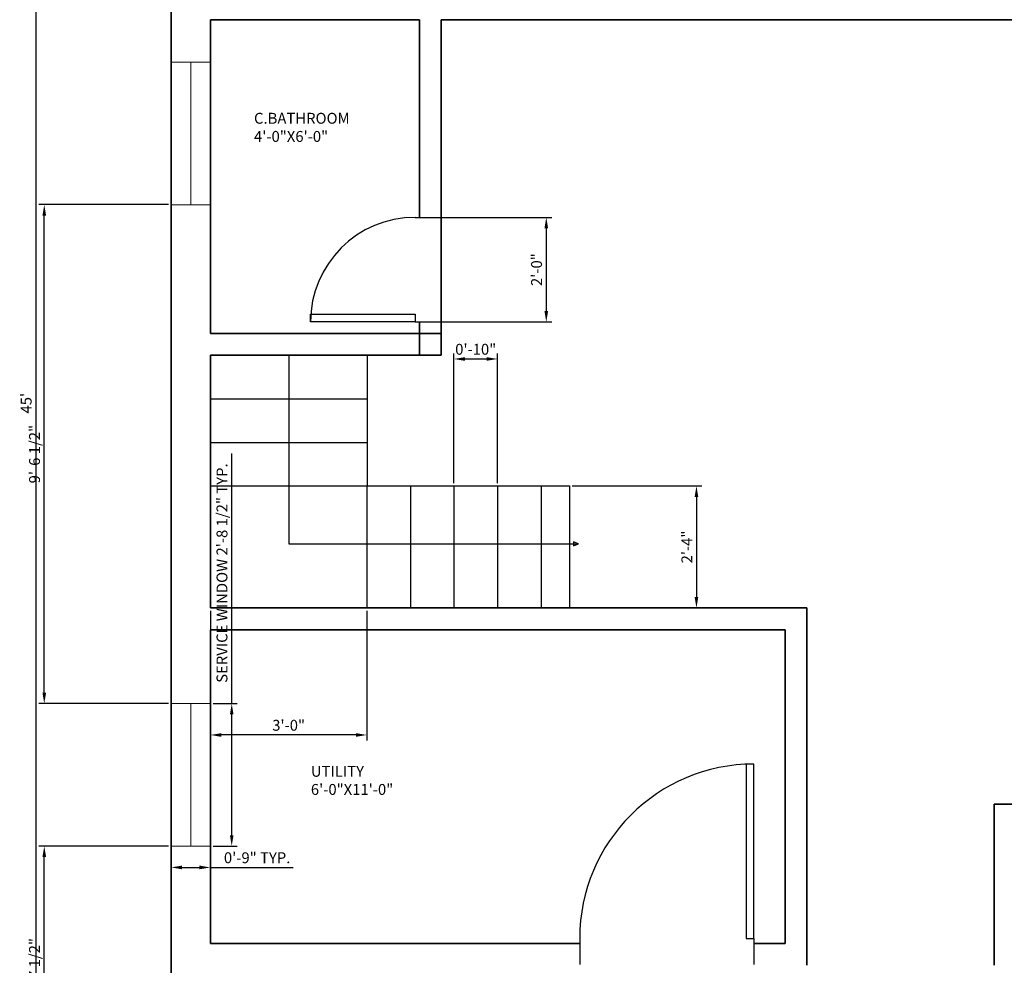
# Model space of a CAD drawing. Units: inches. Extents: x 2981 to 3526, y 1512 to 2158.
# Tile 2 of 4: x 2981 to 3207, y 1713 to 1930. Entities that reach past the tile are written whole.
import ezdxf

# ---------------------------------------------------------------- set-up
doc = ezdxf.new("R2010")
doc.units = ezdxf.units.IN
for name, color, linetype, lineweight in [('A-ANNO-DIMS', 2, 'Continuous', 18), ('A-AREA-IDEN', 7, 'Continuous', 18), ('A-DOOR', 4, 'Continuous', 25), ('A-FLOR-STRS', 7, 'Continuous', 25), ('A-GLAZ', 4, 'Continuous', 18), ('A-WALL', 7, 'Continuous', 35)]:
    doc.layers.add(name, color=color, linetype=linetype, lineweight=lineweight)
doc.styles.get("Standard").update_dxf_attribs({"font": 'arial.ttf'})
doc.dimstyles.new('ISO-25', dxfattribs={"dimtxt": 2.5, "dimasz": 2.5, "dimexe": 1.25, "dimexo": 0.625, "dimtad": 1, "dimlunit": 3, "dimtxsty": 'Standard', "dimcen": 2.5, "dimadec": 0, "dimazin": 0, "dimtfac": 1, "dimtmove": 0, "dimatfit": 3, "dimfxl": 1, "dimarcsym": 0})

# ---------------------------------------------------------------- blocks, each defined once
blk = doc.blocks.new('*U5')
for p, q in [((0, 0), (0, -6)), ((24, 0), (24, -6))]:
    blk.add_line(p, q)
blk.add_lwpolyline([(0, 0), (0, 24), (1.75, 24), (1.75, 0)], close=True)
blk.add_arc((0, 0), 24, 0, 90)
blk = doc.blocks.new('*U4')
for p, q in [((0, 0), (0, -6)), ((-40, 0), (-40, -6))]:
    blk.add_line(p, q)
blk.add_lwpolyline([(0, 0), (0, 40), (-1.75, 40), (-1.75, 0)], close=True)
blk.add_arc((0, 0), 40, 90, 180)
blk = doc.blocks.new('*D15')
at = {"layer": 'A-ANNO-DIMS', "color": 0, "lineweight": -2, "transparency": 16777216}
for p, q in [((3014.77, 2112.2), (2983.05, 2112.2)), ((2984.3, 2109.7), (2984.3, 1574.7)), ((3014.77, 1572.2), (2983.05, 1572.2))]:
    blk.add_line(p, q, dxfattribs=at)
at = {"layer": 'A-ANNO-DIMS', "color": 0, "transparency": 16777216}
for points in [[(2983.89, 2109.7), (2984.72, 2109.7), (2984.3, 2112.2)], [(2983.89, 1574.7), (2984.72, 1574.7), (2984.3, 1572.2)]]:
    blk.add_solid(points, dxfattribs=at)
at = {"layer": 'Defpoints', "color": 0, "transparency": 16777216}
for p in [(3015.4, 2112.2), (2984.3, 1572.2), (3015.4, 1572.2)]:
    blk.add_point(p, dxfattribs=at)
at = {"layer": 'A-ANNO-DIMS', "color": 0, "transparency": 16777216, "insert": (2982.41, 1842.2), "char_height": 2.5, "attachment_point": 5, "rotation": 90}
blk.add_mtext("45'", dxfattribs=at)
blk = doc.blocks.new('WIN-33IN-SERVICE')
for p, q in [((9, 32.7), (0, 32.7)), ((0, 32.7), (0, 0)), ((9, 32.7), (4.5, 32.7)), ((4.5, 32.7), (4.5, 0)), ((9, 0), (9, 32.7)), ((0, 0), (9, 0))]:
    blk.add_line(p, q)
blk = doc.blocks.new('*D33')
at = {"layer": 'A-ANNO-DIMS', "color": 0, "lineweight": -2, "transparency": 16777216}
for p, q in [((3029.3, 1773.26), (3029.3, 1830.66)), ((3025.02, 1773.26), (3030.55, 1773.26)), ((3029.3, 1743.06), (3029.3, 1770.76)), ((3025.02, 1740.56), (3030.55, 1740.56))]:
    blk.add_line(p, q, dxfattribs=at)
at = {"layer": 'A-ANNO-DIMS', "color": 0, "transparency": 16777216}
for points in [[(3028.89, 1770.76), (3029.72, 1770.76), (3029.3, 1773.26)], [(3028.89, 1743.06), (3029.72, 1743.06), (3029.3, 1740.56)]]:
    blk.add_solid(points, dxfattribs=at)
at = {"layer": 'Defpoints', "color": 0, "transparency": 16777216}
for p in [(3024.4, 1773.26), (3029.3, 1773.26), (3024.4, 1740.56)]:
    blk.add_point(p, dxfattribs=at)
at = {"layer": 'A-ANNO-DIMS', "color": 0, "transparency": 16777216, "insert": (3027.39, 1803.21), "char_height": 2.5, "attachment_point": 5, "rotation": 90}
blk.add_mtext('SERVICE WINDOW 2\'-8 1/2" TYP.', dxfattribs=at)
blk = doc.blocks.new('*D34')
at = {"layer": 'A-ANNO-DIMS', "color": 0, "lineweight": -2, "transparency": 16777216}
for p, q in [((3015.4, 1739.94), (3015.4, 1734.41)), ((3024.4, 1739.94), (3024.4, 1734.41)), ((3017.9, 1735.66), (3021.9, 1735.66)), ((3024.4, 1735.66), (3043.39, 1735.66))]:
    blk.add_line(p, q, dxfattribs=at)
at = {"layer": 'A-ANNO-DIMS', "color": 0, "transparency": 16777216}
for points in [[(3017.9, 1736.08), (3017.9, 1735.24), (3015.4, 1735.66)], [(3021.9, 1736.08), (3021.9, 1735.24), (3024.4, 1735.66)]]:
    blk.add_solid(points, dxfattribs=at)
at = {"layer": 'Defpoints', "color": 0, "transparency": 16777216}
for p in [(3015.4, 1740.56), (3024.4, 1740.56), (3024.4, 1735.66)]:
    blk.add_point(p, dxfattribs=at)
at = {"layer": 'A-ANNO-DIMS', "color": 0, "transparency": 16777216, "insert": (3035.14, 1737.56), "char_height": 2.5, "attachment_point": 5}
blk.add_mtext('0\'-9" TYP.', dxfattribs=at)
blk = doc.blocks.new('*D36')
at = {"layer": 'A-ANNO-DIMS', "color": 0, "lineweight": -2, "transparency": 16777216}
for p, q in [((3073.02, 1884.85), (3102.79, 1884.85)), ((3101.54, 1882.35), (3101.54, 1863.35)), ((3073.02, 1860.85), (3102.79, 1860.85))]:
    blk.add_line(p, q, dxfattribs=at)
at = {"layer": 'A-ANNO-DIMS', "color": 0, "transparency": 16777216}
for points in [[(3101.13, 1882.35), (3101.96, 1882.35), (3101.54, 1884.85)], [(3101.13, 1863.35), (3101.96, 1863.35), (3101.54, 1860.85)]]:
    blk.add_solid(points, dxfattribs=at)
at = {"layer": 'Defpoints', "color": 0, "transparency": 16777216}
for p in [(3072.4, 1884.85), (3072.4, 1860.85), (3101.54, 1860.85)]:
    blk.add_point(p, dxfattribs=at)
at = {"layer": 'A-ANNO-DIMS', "color": 0, "transparency": 16777216, "insert": (3099.64, 1872.85), "char_height": 2.5, "attachment_point": 5, "rotation": 90}
blk.add_mtext('2\'-0"', dxfattribs=at)
blk = doc.blocks.new('*D51')
at = {"layer": 'A-ANNO-DIMS', "color": 0, "lineweight": -2, "transparency": 16777216}
for p, q in [((3014.77, 1740.56), (2985, 1740.56)), ((2986.25, 1687.44), (2986.25, 1738.06)), ((3014.77, 1684.94), (2985, 1684.94))]:
    blk.add_line(p, q, dxfattribs=at)
at = {"layer": 'A-ANNO-DIMS', "color": 0, "transparency": 16777216}
for points in [[(2985.84, 1738.06), (2986.67, 1738.06), (2986.25, 1740.56)], [(2985.84, 1687.44), (2986.67, 1687.44), (2986.25, 1684.94)]]:
    blk.add_solid(points, dxfattribs=at)
at = {"layer": 'Defpoints', "color": 0, "transparency": 16777216}
for p in [(2986.25, 1740.56), (3015.4, 1740.56), (3015.4, 1684.94)]:
    blk.add_point(p, dxfattribs=at)
at = {"layer": 'A-ANNO-DIMS', "color": 0, "transparency": 16777216, "insert": (2984.34, 1712.75), "char_height": 2.5, "attachment_point": 5, "rotation": 90}
blk.add_mtext('4\'-7 1/2"', dxfattribs=at)
blk = doc.blocks.new('*D52')
at = {"layer": 'A-ANNO-DIMS', "color": 0, "lineweight": -2, "transparency": 16777216}
for p, q in [((3014.77, 1887.76), (2985, 1887.76)), ((2986.25, 1775.76), (2986.25, 1885.26)), ((3014.77, 1773.26), (2985, 1773.26))]:
    blk.add_line(p, q, dxfattribs=at)
at = {"layer": 'A-ANNO-DIMS', "color": 0, "transparency": 16777216}
for points in [[(2985.84, 1885.26), (2986.67, 1885.26), (2986.25, 1887.76)], [(2985.84, 1775.76), (2986.67, 1775.76), (2986.25, 1773.26)]]:
    blk.add_solid(points, dxfattribs=at)
at = {"layer": 'Defpoints', "color": 0, "transparency": 16777216}
for p in [(2986.25, 1887.76), (3015.4, 1887.76), (3015.4, 1773.26)]:
    blk.add_point(p, dxfattribs=at)
at = {"layer": 'A-ANNO-DIMS', "color": 0, "transparency": 16777216, "insert": (2984.34, 1830.51), "char_height": 2.5, "attachment_point": 5, "rotation": 90}
blk.add_mtext('9\'-6 1/2"', dxfattribs=at)
blk = doc.blocks.new('*D53')
at = {"layer": 'A-ANNO-DIMS', "color": 0, "lineweight": -2, "transparency": 16777216}
for p, q in [((3107.51, 1823.2), (3137.28, 1823.2)), ((3136.03, 1820.7), (3136.03, 1797.7)), ((3107.51, 1795.2), (3137.28, 1795.2))]:
    blk.add_line(p, q, dxfattribs=at)
at = {"layer": 'A-ANNO-DIMS', "color": 0, "transparency": 16777216}
for points in [[(3135.62, 1820.7), (3136.45, 1820.7), (3136.03, 1823.2)], [(3135.62, 1797.7), (3136.45, 1797.7), (3136.03, 1795.2)]]:
    blk.add_solid(points, dxfattribs=at)
at = {"layer": 'Defpoints', "color": 0, "transparency": 16777216}
for p in [(3106.89, 1823.2), (3106.89, 1795.2), (3136.03, 1795.2)]:
    blk.add_point(p, dxfattribs=at)
at = {"layer": 'A-ANNO-DIMS', "color": 0, "transparency": 16777216, "insert": (3134.15, 1809.2), "char_height": 2.5, "attachment_point": 5, "rotation": 90}
blk.add_mtext('2\'-4"', dxfattribs=at)
blk = doc.blocks.new('*D54')
at = {"layer": 'A-ANNO-DIMS', "color": 0, "lineweight": -2, "transparency": 16777216}
for p, q in [((3024.4, 1794.58), (3024.4, 1764.81)), ((3060.34, 1794.58), (3060.34, 1764.81)), ((3057.84, 1766.06), (3026.9, 1766.06))]:
    blk.add_line(p, q, dxfattribs=at)
at = {"layer": 'A-ANNO-DIMS', "color": 0, "transparency": 16777216}
for points in [[(3026.9, 1766.47), (3026.9, 1765.64), (3024.4, 1766.06)], [(3057.84, 1766.47), (3057.84, 1765.64), (3060.34, 1766.06)]]:
    blk.add_solid(points, dxfattribs=at)
at = {"layer": 'Defpoints', "color": 0, "transparency": 16777216}
for p in [(3024.4, 1795.2), (3060.34, 1795.2), (3024.4, 1766.06)]:
    blk.add_point(p, dxfattribs=at)
at = {"layer": 'A-ANNO-DIMS', "color": 0, "transparency": 16777216, "insert": (3042.37, 1767.96), "char_height": 2.5, "attachment_point": 5}
blk.add_mtext('3\'-0"', dxfattribs=at)
blk = doc.blocks.new('*D55')
at = {"layer": 'A-ANNO-DIMS', "color": 0, "lineweight": -2, "transparency": 16777216}
for p, q in [((3080.34, 1823.83), (3080.34, 1853.6)), ((3082.84, 1852.35), (3087.84, 1852.35)), ((3090.34, 1823.83), (3090.34, 1853.6))]:
    blk.add_line(p, q, dxfattribs=at)
at = {"layer": 'A-ANNO-DIMS', "color": 0, "transparency": 16777216}
for points in [[(3082.84, 1852.76), (3082.84, 1851.93), (3080.34, 1852.35)], [(3087.84, 1852.76), (3087.84, 1851.93), (3090.34, 1852.35)]]:
    blk.add_solid(points, dxfattribs=at)
at = {"layer": 'Defpoints', "color": 0, "transparency": 16777216}
for p in [(3090.34, 1852.35), (3080.34, 1823.2), (3090.34, 1823.2)]:
    blk.add_point(p, dxfattribs=at)
at = {"layer": 'A-ANNO-DIMS', "color": 0, "transparency": 16777216, "insert": (3085.34, 1854.25), "char_height": 2.5, "attachment_point": 5}
blk.add_mtext('0\'-10"', dxfattribs=at)

msp = doc.modelspace()

# ---------------------------------------------------------------- linework, layer by layer
at = {"layer": 'A-FLOR-STRS'}
for p, q in [((3024.399, 1853.202), (3060.399, 1853.202)), ((3042.399, 1853.202), (3042.399, 1809.935)), ((3060.399, 1853.202), (3060.399, 1823.202)), ((3024.399, 1843.202), (3060.399, 1843.202)), ((3024.399, 1833.202), (3060.399, 1833.202)), ((3024.399, 1823.202), (3060.399, 1823.202)), ((3060.345, 1823.202), (3060.345, 1795.202)), ((3060.399, 1823.202), (3106.89, 1823.202)), ((3070.345, 1823.202), (3070.345, 1795.202)), ((3080.345, 1823.202), (3080.345, 1795.202)), ((3090.345, 1823.202), (3090.345, 1795.202)), ((3100.345, 1823.202), (3100.345, 1795.202)), ((3106.89, 1823.202), (3106.89, 1795.202)), ((3042.399, 1809.935), (3108.912, 1809.935)), ((3107.789, 1810.388), (3107.789, 1809.456)), ((3108.912, 1809.935), (3107.789, 1810.388)), ((3107.789, 1809.456), (3108.912, 1809.935))]:
    msp.add_line(p, q, dxfattribs=at)
at = {"layer": 'A-WALL'}
for p, q in [((3015.399, 1572.202), (3015.399, 2112.202)), ((3024.399, 1930.202), (3072.399, 1930.202)), ((3024.399, 1930.202), (3072.399, 1930.202)), ((3024.399, 1858.202), (3024.399, 1930.202)), ((3072.399, 1884.85), (3072.399, 1930.202)), ((3077.399, 1853.202), (3077.399, 1930.202)), ((3077.399, 1930.202), (3216.399, 1930.202)), ((3077.399, 1930.202), (3221.399, 1930.202)), ((3072.399, 1853.202), (3072.399, 1860.85)), ((3024.399, 1858.202), (3077.399, 1858.202)), ((3024.399, 1853.202), (3077.399, 1853.202)), ((3024.399, 1795.202), (3024.399, 1853.202)), ((3161.399, 1795.202), (3024.399, 1795.202)), ((3161.399, 1713.202), (3161.399, 1795.202)), ((3156.399, 1790.202), (3024.399, 1790.202)), ((3024.399, 1718.202), (3024.399, 1790.202)), ((3156.399, 1718.202), (3156.399, 1790.202)), ((3204.399, 1745.202), (3204.399, 1750.202)), ((3204.399, 1750.202), (3209.399, 1750.202)), ((3204.399, 1713.202), (3204.399, 1745.202)), ((3109.227, 1718.202), (3024.399, 1718.202)), ((3156.399, 1718.202), (3149.227, 1718.202))]:
    msp.add_line(p, q, dxfattribs=at)

# ---------------------------------------------------------------- block references
at = {"layer": 'A-DOOR', "rotation": 89.99999999999999}
msp.add_blockref('*U5', (3071.401, 1860.85), dxfattribs=at)
at = {"layer": 'A-DOOR'}
msp.add_blockref('*U4', (3149.227, 1719.388), dxfattribs=at)
at = {"layer": 'A-GLAZ'}
for p in [(3015.399, 1887.757), (3015.399, 1740.564)]:
    msp.add_blockref('WIN-33IN-SERVICE', p, dxfattribs=at)

# ---------------------------------------------------------------- texts
at = {"layer": 'A-AREA-IDEN', "char_height": 2.5, "attachment_point": 1}
for s, width, insert in [('C.BATHROOM\\P4\'-0"X6\'-0"', 21.8805, (3034.423, 1908.837)), ('UTILITY\\P6\'-0"X11\'-0"', 45.34657, (3047.483, 1758.974))]:
    msp.add_mtext_dynamic_manual_height_columns(s, width=width, gutter_width=12.5, heights=[0], dxfattribs=dict(at, insert=insert))

# ---------------------------------------------------------------- dimensions: what is measured, and where the dimension line sits
at = {"layer": 'A-ANNO-DIMS'}
for base, p1, p2, angle, override, picture, middle in [((2984.303, 1572.202), (3015.399, 2112.202), (3015.399, 1572.202), 90, {"dimclrd": 0, "dimclre": 0, "dimclrt": 0}, '*D15', (2982.407, 1842.202)), ((2986.254, 1887.757), (3015.399, 1773.263), (3015.399, 1887.757), 90, {"dimdec": 1, "dimlfac": 1, "dimrnd": 0, "dimzin": 1, "dimdsep": 46, "dimlunit": 4, "dimfrac": 2}, '*D52', (2984.337, 1830.51)), ((3101.544, 1860.85), (3072.399, 1884.85), (3072.399, 1860.85), 270, {"dimdec": 1, "dimlfac": 1, "dimrnd": 0, "dimzin": 1, "dimdsep": 46, "dimlunit": 4, "dimfrac": 2}, '*D36', (3099.643, 1872.85)), ((3136.035, 1795.202), (3106.89, 1823.202), (3106.89, 1795.202), 270, {"dimdec": 1, "dimlfac": 1, "dimrnd": 0, "dimzin": 1, "dimdsep": 46, "dimlunit": 4, "dimfrac": 2}, '*D53', (3134.154, 1809.202)), ((3024.399, 1766.057), (3060.345, 1795.202), (3024.399, 1795.202), 180, {"dimdec": 1, "dimlfac": 1, "dimrnd": 0, "dimzin": 1, "dimdsep": 46, "dimlunit": 4, "dimfrac": 2}, '*D54', (3042.372, 1767.96)), ((2986.254, 1740.564), (3015.399, 1684.94), (3015.399, 1740.564), 90, {"dimdec": 1, "dimlfac": 1, "dimrnd": 0, "dimzin": 1, "dimdsep": 46, "dimlunit": 4, "dimfrac": 2}, '*D51', (2984.337, 1712.752))]:
    dim = msp.add_linear_dim(base=base, p1=p1, p2=p2, angle=angle, dimstyle='ISO-25', override=override, dxfattribs=at)
    dim.commit()
    dim.dimension.update_dxf_attribs({"geometry": picture, "text_midpoint": middle})
dim = msp.add_linear_dim(base=(3090.345, 1852.347), p1=(3080.345, 1823.202), p2=(3090.345, 1823.202), dimstyle='ISO-25', override={"dimdec": 1, "dimlfac": 1, "dimrnd": 0, "dimzin": 1, "dimdsep": 46, "dimlunit": 4, "dimfrac": 2}, dxfattribs=at)
dim.commit()
dim.dimension.update_dxf_attribs({"geometry": '*D55', "text_midpoint": (3085.345, 1854.249)})
dim = msp.add_linear_dim(base=(3029.304, 1773.263), p1=(3024.399, 1740.564), p2=(3024.399, 1773.263), angle=90, text='SERVICE WINDOW <> TYP.', dimstyle='ISO-25', override={"dimdec": 1, "dimlfac": 1, "dimrnd": 0, "dimzin": 1, "dimdsep": 46, "dimlunit": 4, "dimfrac": 2}, dxfattribs=at)
dim.commit()
dim.dimension.update_dxf_attribs({"geometry": '*D33', "text_midpoint": (3027.386, 1803.213)})
dim = msp.add_linear_dim(base=(3024.399, 1735.659), p1=(3015.399, 1740.564), p2=(3024.399, 1740.564), text='<> TYP.', dimstyle='ISO-25', override={"dimdec": 1, "dimlfac": 1, "dimrnd": 0, "dimzin": 1, "dimdsep": 46, "dimlunit": 4, "dimfrac": 2}, dxfattribs=at)
dim.commit()
dim.dimension.update_dxf_attribs({"geometry": '*D34', "text_midpoint": (3035.144, 1737.56)})

doc.saveas('drawing.dxf')
